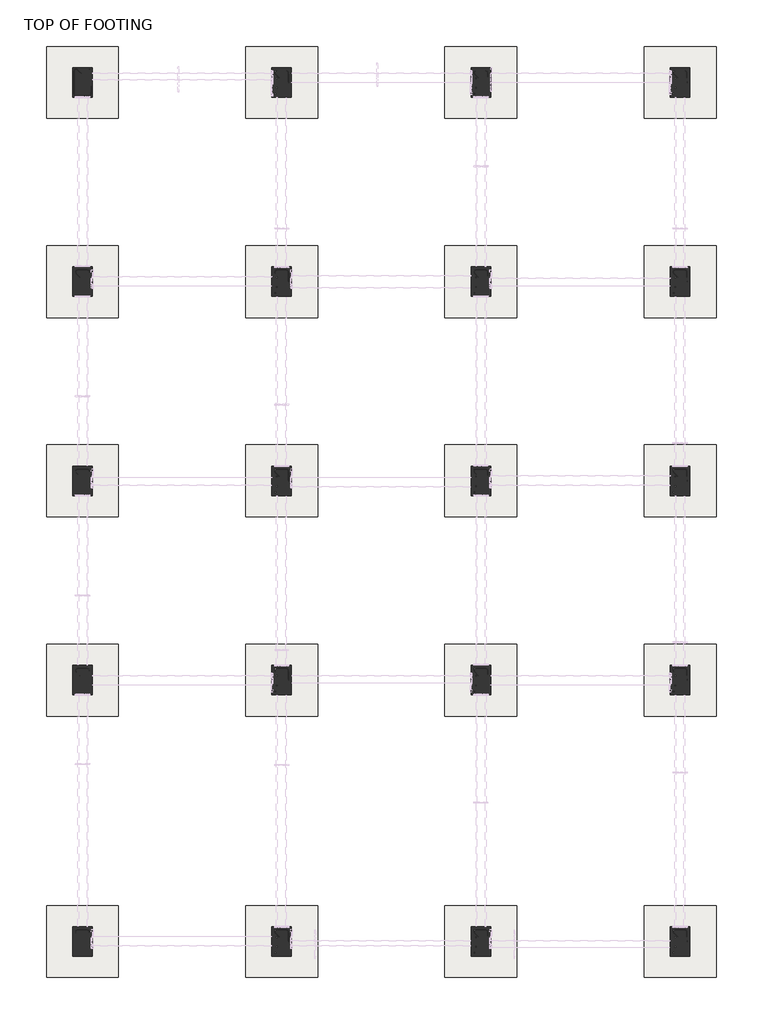
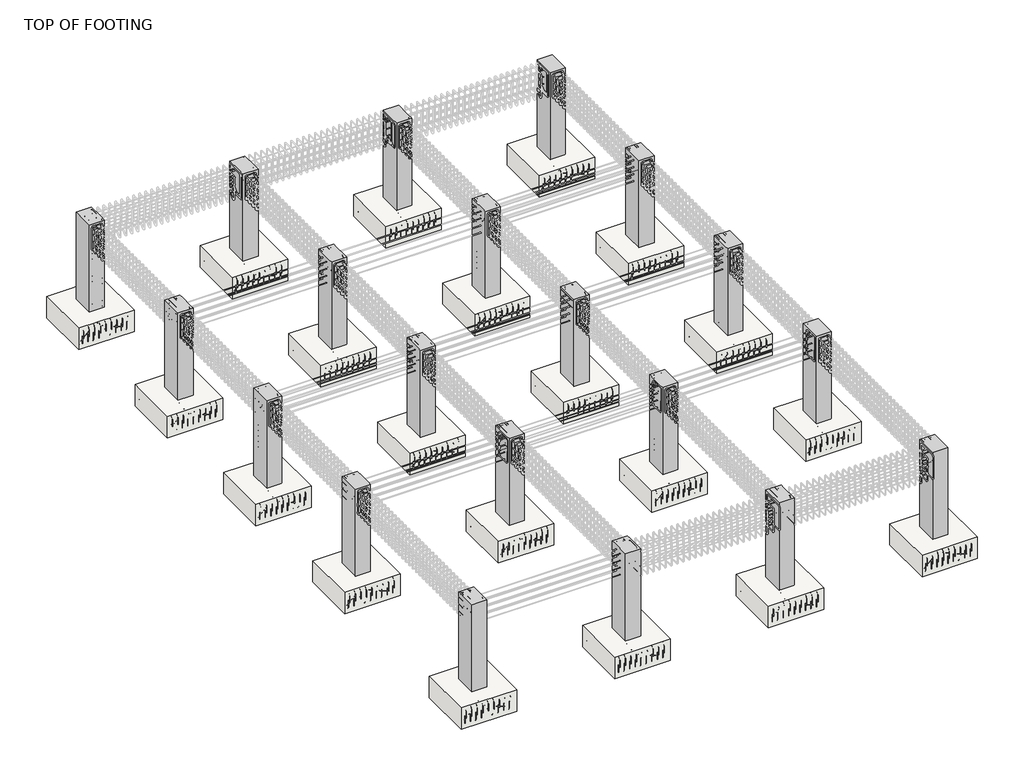
# One storey, part 1 of 18: 20 columns, 20 slabs.
"""IFC4 building model written with IfcOpenShell, lengths in millimetres."""

from ifc_helpers import new_model, si_unit, origin, place, context, project, spatial, faceted_brep, transform, mapped, element, save
from components import m_footing_rectangular_1100mm_x_1100mm_x_450mm_64323a20

model = new_model("IFC4")

# Units and contexts
model_context = context("Model", 3, world=origin())
ifc_project = project(units=[si_unit("LENGTHUNIT", "METRE", prefix="MILLI")], contexts=[model_context])

# Site, building, storey
site = spatial("IfcSite", under=ifc_project)
building = spatial("IfcBuilding", under=site)
storey = spatial("IfcBuildingStorey", under=building, Name="TOP OF FOOTING", Elevation=-1828.8)

# Columns
placement = place(None, origin())
element("IfcColumn", 1, ObjectType="M_Concrete-Rectangular-Column : 300 x 450mm", at=placement, inside=storey, context=model_context, shape_type="Brep", body=[
    faceted_brep([(-10892.3067643, 19025.6598681, -1828.8), (-10892.3067643, 18575.6598681, -1828.8), (-11192.3067643, 18575.6598681, -1828.8), (-11192.3067643, 19025.6598681, -1828.8), (-10892.3067643, 19025.6598681, 0.0), (-10892.3067643, 18725.6598681, 0.0), (-10892.3067643, 18575.6598681, 0.0), (-11192.3067643, 18575.6598681, 0.0), (-11192.3067643, 19025.6598681, 0.0)], [[[0, 1, 2, 3]], [[4, 5, 6, 1, 0]], [[6, 7, 2, 1]], [[7, 8, 3, 2]], [[8, 4, 0, 3]], [[4, 8, 7, 6, 5]]]),
])
element("IfcColumn", 2, ObjectType="M_Concrete-Rectangular-Column : 300 x 450mm", at=placement, inside=storey, context=model_context, shape_type="Brep", body=[
    faceted_brep([(-7844.3067643, 19025.6598681, -1828.8), (-7844.3067643, 18575.6598681, -1828.8), (-8144.3067643, 18575.6598681, -1828.8), (-8144.3067643, 19025.6598681, -1828.8), (-7844.3067643, 19025.6598681, 0.0), (-7844.3067643, 18725.6598681, 0.0), (-7844.3067643, 18575.6598681, 0.0), (-8144.3067643, 18575.6598681, 0.0), (-8144.3067643, 18725.6598681, 0.0), (-8144.3067643, 19025.6598681, 0.0)], [[[0, 1, 2, 3]], [[4, 5, 6, 1, 0]], [[6, 7, 2, 1]], [[7, 8, 9, 3, 2]], [[9, 4, 0, 3]], [[4, 9, 8, 7, 6, 5]]]),
])
element("IfcColumn", 3, ObjectType="M_Concrete-Rectangular-Column : 300 x 450mm", at=placement, inside=storey, context=model_context, shape_type="Brep", body=[
    faceted_brep([(-4796.3067643, 19025.6598681, -1828.8), (-4796.3067643, 18575.6598681, -1828.8), (-5096.3067643, 18575.6598681, -1828.8), (-5096.3067643, 19025.6598681, -1828.8), (-4796.3067643, 19025.6598681, 0.0), (-4796.3067643, 18725.6598681, 0.0), (-4796.3067643, 18575.6598681, 0.0), (-5096.3067643, 18575.6598681, 0.0), (-5096.3067643, 18725.6598681, 0.0), (-5096.3067643, 19025.6598681, 0.0)], [[[0, 1, 2, 3]], [[4, 5, 6, 1, 0]], [[6, 7, 2, 1]], [[7, 8, 9, 3, 2]], [[9, 4, 0, 3]], [[4, 9, 8, 7, 6, 5]]]),
])
element("IfcColumn", 4, ObjectType="M_Concrete-Rectangular-Column : 300 x 450mm", at=placement, inside=storey, context=model_context, shape_type="Brep", body=[
    faceted_brep([(-1748.3067643, 19025.6598681, -1828.8), (-1748.3067643, 18575.6598681, -1828.8), (-2048.3067643, 18575.6598681, -1828.8), (-2048.3067643, 19025.6598681, -1828.8), (-1748.3067643, 19025.6598681, 0.0), (-1748.3067643, 18575.6598681, 0.0), (-2048.3067643, 18575.6598681, 0.0), (-2048.3067643, 18725.6598681, 0.0), (-2048.3067643, 19025.6598681, 0.0)], [[[0, 1, 2, 3]], [[4, 5, 1, 0]], [[5, 6, 2, 1]], [[6, 7, 8, 3, 2]], [[8, 4, 0, 3]], [[4, 8, 7, 6, 5]]]),
])
element("IfcColumn", 5, ObjectType="M_Concrete-Rectangular-Column : 300 x 450mm", at=placement, inside=storey, context=model_context, shape_type="Brep", body=[
    faceted_brep([(-1748.3067643, 15977.6598681, -1828.8), (-1748.3067643, 15527.6598681, -1828.8), (-2048.3067643, 15527.6598681, -1828.8), (-2048.3067643, 15977.6598681, -1828.8), (-1748.3067643, 15977.6598681, 0.0), (-1748.3067643, 15527.6598681, 0.0), (-2048.3067643, 15527.6598681, 0.0), (-2048.3067643, 15602.6598681, 0.0), (-2048.3067643, 15902.6598681, 0.0), (-2048.3067643, 15977.6598681, 0.0)], [[[0, 1, 2, 3]], [[4, 5, 1, 0]], [[5, 6, 2, 1]], [[6, 7, 8, 9, 3, 2]], [[9, 4, 0, 3]], [[4, 9, 8, 7, 6, 5]]]),
])
element("IfcColumn", 6, ObjectType="M_Concrete-Rectangular-Column : 300 x 450mm", at=placement, inside=storey, context=model_context, shape_type="Brep", body=[
    faceted_brep([(-4796.3067643, 15977.6598681, -1828.8), (-4796.3067643, 15527.6598681, -1828.8), (-5096.3067643, 15527.6598681, -1828.8), (-5096.3067643, 15977.6598681, -1828.8), (-4796.3067643, 15977.6598681, 0.0), (-4796.3067643, 15902.6598681, 0.0), (-4796.3067643, 15602.6598681, 0.0), (-4796.3067643, 15527.6598681, 0.0), (-5096.3067643, 15527.6598681, 0.0), (-5096.3067643, 15602.6598681, 0.0), (-5096.3067643, 15902.6598681, 0.0), (-5096.3067643, 15977.6598681, 0.0)], [[[0, 1, 2, 3]], [[4, 5, 6, 7, 1, 0]], [[7, 8, 2, 1]], [[8, 9, 10, 11, 3, 2]], [[11, 4, 0, 3]], [[4, 11, 10, 9, 8, 7, 6, 5]]]),
])
element("IfcColumn", 7, ObjectType="M_Concrete-Rectangular-Column : 300 x 450mm", at=placement, inside=storey, context=model_context, shape_type="Brep", body=[
    faceted_brep([(-7844.3067643, 15977.6598681, -1828.8), (-7844.3067643, 15527.6598681, -1828.8), (-8144.3067643, 15527.6598681, -1828.8), (-8144.3067643, 15977.6598681, -1828.8), (-7844.3067643, 15977.6598681, 0.0), (-7844.3067643, 15902.6598681, 0.0), (-7844.3067643, 15602.6598681, 0.0), (-7844.3067643, 15527.6598681, 0.0), (-8144.3067643, 15527.6598681, 0.0), (-8144.3067643, 15602.6598681, 0.0), (-8144.3067643, 15902.6598681, 0.0), (-8144.3067643, 15977.6598681, 0.0)], [[[0, 1, 2, 3]], [[4, 5, 6, 7, 1, 0]], [[7, 8, 2, 1]], [[8, 9, 10, 11, 3, 2]], [[11, 4, 0, 3]], [[4, 11, 10, 9, 8, 7, 6, 5]]]),
])
element("IfcColumn", 8, ObjectType="M_Concrete-Rectangular-Column : 300 x 450mm", at=placement, inside=storey, context=model_context, shape_type="Brep", body=[
    faceted_brep([(-10892.3067643, 15977.6598681, -1828.8), (-10892.3067643, 15527.6598681, -1828.8), (-11192.3067643, 15527.6598681, -1828.8), (-11192.3067643, 15977.6598681, -1828.8), (-10892.3067643, 15977.6598681, 0.0), (-10892.3067643, 15902.6598681, 0.0), (-10892.3067643, 15602.6598681, 0.0), (-10892.3067643, 15527.6598681, 0.0), (-11192.3067643, 15527.6598681, 0.0), (-11192.3067643, 15977.6598681, 0.0)], [[[0, 1, 2, 3]], [[4, 5, 6, 7, 1, 0]], [[7, 8, 2, 1]], [[8, 9, 3, 2]], [[9, 4, 0, 3]], [[4, 9, 8, 7, 6, 5]]]),
])
element("IfcColumn", 9, ObjectType="M_Concrete-Rectangular-Column : 300 x 450mm", at=placement, inside=storey, context=model_context, shape_type="Brep", body=[
    faceted_brep([(-10892.3067643, 12929.6598681, -1828.8), (-10892.3067643, 12479.6598681, -1828.8), (-11192.3067643, 12479.6598681, -1828.8), (-11192.3067643, 12929.6598681, -1828.8), (-10892.3067643, 12929.6598681, 0.0), (-10892.3067643, 12779.6598681, 0.0), (-10892.3067643, 12554.6598681, 0.0), (-10892.3067643, 12479.6598681, 0.0), (-11192.3067643, 12479.6598681, 0.0), (-11192.3067643, 12929.6598681, 0.0)], [[[0, 1, 2, 3]], [[4, 5, 6, 7, 1, 0]], [[7, 8, 2, 1]], [[8, 9, 3, 2]], [[9, 4, 0, 3]], [[4, 9, 8, 7, 6, 5]]]),
])
element("IfcColumn", 10, ObjectType="M_Concrete-Rectangular-Column : 300 x 450mm", at=placement, inside=storey, context=model_context, shape_type="Brep", body=[
    faceted_brep([(-7844.3067643, 12929.6598681, -1828.8), (-7844.3067643, 12479.6598681, -1828.8), (-8144.3067643, 12479.6598681, -1828.8), (-8144.3067643, 12929.6598681, -1828.8), (-7844.3067643, 12929.6598681, 0.0), (-7844.3067643, 12779.6598681, 0.0), (-7844.3067643, 12554.6598681, 0.0), (-7844.3067643, 12479.6598681, 0.0), (-8144.3067643, 12479.6598681, 0.0), (-8144.3067643, 12554.6598681, 0.0), (-8144.3067643, 12779.6598681, 0.0), (-8144.3067643, 12929.6598681, 0.0)], [[[0, 1, 2, 3]], [[4, 5, 6, 7, 1, 0]], [[7, 8, 2, 1]], [[8, 9, 10, 11, 3, 2]], [[11, 4, 0, 3]], [[4, 11, 10, 9, 8, 7, 6, 5]]]),
])
element("IfcColumn", 11, ObjectType="M_Concrete-Rectangular-Column : 300 x 450mm", at=placement, inside=storey, context=model_context, shape_type="Brep", body=[
    faceted_brep([(-4796.3067643, 12929.6598681, -1828.8), (-4796.3067643, 12479.6598681, -1828.8), (-5096.3067643, 12479.6598681, -1828.8), (-5096.3067643, 12929.6598681, -1828.8), (-4796.3067643, 12929.6598681, 0.0), (-4796.3067643, 12779.6598681, 0.0), (-4796.3067643, 12554.6598681, 0.0), (-4796.3067643, 12479.6598681, 0.0), (-5096.3067643, 12479.6598681, 0.0), (-5096.3067643, 12554.6598681, 0.0), (-5096.3067643, 12779.6598681, 0.0), (-5096.3067643, 12929.6598681, 0.0)], [[[0, 1, 2, 3]], [[4, 5, 6, 7, 1, 0]], [[7, 8, 2, 1]], [[8, 9, 10, 11, 3, 2]], [[11, 4, 0, 3]], [[4, 11, 10, 9, 8, 7, 6, 5]]]),
])
element("IfcColumn", 12, ObjectType="M_Concrete-Rectangular-Column : 300 x 450mm", at=placement, inside=storey, context=model_context, shape_type="Brep", body=[
    faceted_brep([(-1748.3067643, 12929.6598681, -1828.8), (-1748.3067643, 12479.6598681, -1828.8), (-2048.3067643, 12479.6598681, -1828.8), (-2048.3067643, 12929.6598681, -1828.8), (-1748.3067643, 12929.6598681, 0.0), (-1748.3067643, 12479.6598681, 0.0), (-2048.3067643, 12479.6598681, 0.0), (-2048.3067643, 12554.6598681, 0.0), (-2048.3067643, 12779.6598681, 0.0), (-2048.3067643, 12929.6598681, 0.0)], [[[0, 1, 2, 3]], [[4, 5, 1, 0]], [[5, 6, 2, 1]], [[6, 7, 8, 9, 3, 2]], [[9, 4, 0, 3]], [[4, 9, 8, 7, 6, 5]]]),
])
element("IfcColumn", 13, ObjectType="M_Concrete-Rectangular-Column : 300 x 450mm", at=placement, inside=storey, context=model_context, shape_type="Brep", body=[
    faceted_brep([(-1748.3067643, 9881.6598681, -1828.8), (-1748.3067643, 9431.6598681, -1828.8), (-2048.3067643, 9431.6598681, -1828.8), (-2048.3067643, 9881.6598681, -1828.8), (-1748.3067643, 9881.6598681, 0.0), (-1748.3067643, 9431.6598681, 0.0), (-2048.3067643, 9431.6598681, 0.0), (-2048.3067643, 9506.6598681, 0.0), (-2048.3067643, 9731.6598681, 0.0), (-2048.3067643, 9881.6598681, 0.0)], [[[0, 1, 2, 3]], [[4, 5, 1, 0]], [[5, 6, 2, 1]], [[6, 7, 8, 9, 3, 2]], [[9, 4, 0, 3]], [[4, 9, 8, 7, 6, 5]]]),
])
element("IfcColumn", 14, ObjectType="M_Concrete-Rectangular-Column : 300 x 450mm", at=placement, inside=storey, context=model_context, shape_type="Brep", body=[
    faceted_brep([(-4796.3067643, 9881.6598681, -1828.8), (-4796.3067643, 9431.6598681, -1828.8), (-5096.3067643, 9431.6598681, -1828.8), (-5096.3067643, 9881.6598681, -1828.8), (-4796.3067643, 9881.6598681, 0.0), (-4796.3067643, 9731.6598681, 0.0), (-4796.3067643, 9506.6598681, 0.0), (-4796.3067643, 9431.6598681, 0.0), (-5096.3067643, 9431.6598681, 0.0), (-5096.3067643, 9506.6598681, 0.0), (-5096.3067643, 9731.6598681, 0.0), (-5096.3067643, 9881.6598681, 0.0)], [[[0, 1, 2, 3]], [[4, 5, 6, 7, 1, 0]], [[7, 8, 2, 1]], [[8, 9, 10, 11, 3, 2]], [[11, 4, 0, 3]], [[4, 11, 10, 9, 8, 7, 6, 5]]]),
])
element("IfcColumn", 15, ObjectType="M_Concrete-Rectangular-Column : 300 x 450mm", at=placement, inside=storey, context=model_context, shape_type="Brep", body=[
    faceted_brep([(-7844.3067643, 9881.6598681, -1828.8), (-7844.3067643, 9431.6598681, -1828.8), (-8144.3067643, 9431.6598681, -1828.8), (-8144.3067643, 9881.6598681, -1828.8), (-7844.3067643, 9881.6598681, 0.0), (-7844.3067643, 9731.6598681, 0.0), (-7844.3067643, 9506.6598681, 0.0), (-7844.3067643, 9431.6598681, 0.0), (-8144.3067643, 9431.6598681, 0.0), (-8144.3067643, 9506.6598681, 0.0), (-8144.3067643, 9731.6598681, 0.0), (-8144.3067643, 9881.6598681, 0.0)], [[[0, 1, 2, 3]], [[4, 5, 6, 7, 1, 0]], [[7, 8, 2, 1]], [[8, 9, 10, 11, 3, 2]], [[11, 4, 0, 3]], [[4, 11, 10, 9, 8, 7, 6, 5]]]),
])
element("IfcColumn", 16, ObjectType="M_Concrete-Rectangular-Column : 300 x 450mm", at=placement, inside=storey, context=model_context, shape_type="Brep", body=[
    faceted_brep([(-10892.3067643, 9881.6598681, -1828.8), (-10892.3067643, 9431.6598681, -1828.8), (-11192.3067643, 9431.6598681, -1828.8), (-11192.3067643, 9881.6598681, -1828.8), (-10892.3067643, 9881.6598681, 0.0), (-10892.3067643, 9731.6598681, 0.0), (-10892.3067643, 9506.6598681, 0.0), (-10892.3067643, 9431.6598681, 0.0), (-11192.3067643, 9431.6598681, 0.0), (-11192.3067643, 9881.6598681, 0.0)], [[[0, 1, 2, 3]], [[4, 5, 6, 7, 1, 0]], [[7, 8, 2, 1]], [[8, 9, 3, 2]], [[9, 4, 0, 3]], [[4, 9, 8, 7, 6, 5]]]),
])
element("IfcColumn", 17, ObjectType="M_Concrete-Rectangular-Column : 300 x 450mm", at=placement, inside=storey, context=model_context, shape_type="Brep", body=[
    faceted_brep([(-10892.3067643, 5881.6598681, -1828.8), (-10892.3067643, 5431.6598681, -1828.8), (-11192.3067643, 5431.6598681, -1828.8), (-11192.3067643, 5881.6598681, -1828.8), (-10892.3067643, 5881.6598681, 0.0), (-10892.3067643, 5806.6598681, 0.0), (-10892.3067643, 5431.6598681, 0.0), (-11192.3067643, 5431.6598681, 0.0), (-11192.3067643, 5881.6598681, 0.0)], [[[0, 1, 2, 3]], [[4, 5, 6, 1, 0]], [[6, 7, 2, 1]], [[7, 8, 3, 2]], [[8, 4, 0, 3]], [[4, 8, 7, 6, 5]]]),
])
element("IfcColumn", 18, ObjectType="M_Concrete-Rectangular-Column : 300 x 450mm", at=placement, inside=storey, context=model_context, shape_type="Brep", body=[
    faceted_brep([(-7844.3067643, 5881.6598681, -1828.8), (-7844.3067643, 5431.6598681, -1828.8), (-8144.3067643, 5431.6598681, -1828.8), (-8144.3067643, 5881.6598681, -1828.8), (-7844.3067643, 5881.6598681, 0.0), (-7844.3067643, 5806.6598681, 0.0), (-7844.3067643, 5431.6598681, 0.0), (-8144.3067643, 5431.6598681, 0.0), (-8144.3067643, 5806.6598681, 0.0), (-8144.3067643, 5881.6598681, 0.0)], [[[0, 1, 2, 3]], [[4, 5, 6, 1, 0]], [[6, 7, 2, 1]], [[7, 8, 9, 3, 2]], [[9, 4, 0, 3]], [[4, 9, 8, 7, 6, 5]]]),
])
element("IfcColumn", 19, ObjectType="M_Concrete-Rectangular-Column : 300 x 450mm", at=placement, inside=storey, context=model_context, shape_type="Brep", body=[
    faceted_brep([(-4796.3067643, 5881.6598681, -1828.8), (-4796.3067643, 5431.6598681, -1828.8), (-5096.3067643, 5431.6598681, -1828.8), (-5096.3067643, 5881.6598681, -1828.8), (-4796.3067643, 5881.6598681, 0.0), (-4796.3067643, 5806.6598681, 0.0), (-4796.3067643, 5431.6598681, 0.0), (-5096.3067643, 5431.6598681, 0.0), (-5096.3067643, 5806.6598681, 0.0), (-5096.3067643, 5881.6598681, 0.0)], [[[0, 1, 2, 3]], [[4, 5, 6, 1, 0]], [[6, 7, 2, 1]], [[7, 8, 9, 3, 2]], [[9, 4, 0, 3]], [[4, 9, 8, 7, 6, 5]]]),
])
element("IfcColumn", 20, ObjectType="M_Concrete-Rectangular-Column : 300 x 450mm", at=placement, inside=storey, context=model_context, shape_type="Brep", body=[
    faceted_brep([(-1748.3067643, 5881.6598681, -1828.8), (-1748.3067643, 5431.6598681, -1828.8), (-2048.3067643, 5431.6598681, -1828.8), (-2048.3067643, 5881.6598681, -1828.8), (-1748.3067643, 5881.6598681, 0.0), (-1748.3067643, 5431.6598681, 0.0), (-2048.3067643, 5431.6598681, 0.0), (-2048.3067643, 5806.6598681, 0.0), (-2048.3067643, 5881.6598681, 0.0)], [[[0, 1, 2, 3]], [[4, 5, 1, 0]], [[5, 6, 2, 1]], [[6, 7, 8, 3, 2]], [[8, 4, 0, 3]], [[4, 8, 7, 6, 5]]]),
])

# Slabs
m_footing_rectangular_1100mm_x_1100mm_x_450mm_shape = m_footing_rectangular_1100mm_x_1100mm_x_450mm_64323a20(model_context)
element("IfcSlab", 21, ObjectType="M_Footing-Rectangular : 1100MM X 1100MM X 450MM", at=placement, inside=storey, context=model_context, shape_type="MappedRepresentation", body=[
    mapped(m_footing_rectangular_1100mm_x_1100mm_x_450mm_shape, transform((-11042.3067643, 18800.6598681, -1828.8), x_axis=(1.0, 0.0, 0.0), y_axis=(0.0, 1.0, 0.0), z_axis=(0.0, 0.0, 1.0))),
])
element("IfcSlab", 22, ObjectType="M_Footing-Rectangular : 1100MM X 1100MM X 450MM", at=placement, inside=storey, context=model_context, shape_type="MappedRepresentation", body=[
    mapped(m_footing_rectangular_1100mm_x_1100mm_x_450mm_shape, transform((-7994.3067643, 18800.6598681, -1828.8), x_axis=(1.0, 0.0, 0.0), y_axis=(0.0, 1.0, 0.0), z_axis=(0.0, 0.0, 1.0))),
])
element("IfcSlab", 23, ObjectType="M_Footing-Rectangular : 1100MM X 1100MM X 450MM", at=placement, inside=storey, context=model_context, shape_type="MappedRepresentation", body=[
    mapped(m_footing_rectangular_1100mm_x_1100mm_x_450mm_shape, transform((-4946.3067643, 18800.6598681, -1828.8), x_axis=(1.0, 0.0, 0.0), y_axis=(0.0, 1.0, 0.0), z_axis=(0.0, 0.0, 1.0))),
])
element("IfcSlab", 24, ObjectType="M_Footing-Rectangular : 1100MM X 1100MM X 450MM", at=placement, inside=storey, context=model_context, shape_type="MappedRepresentation", body=[
    mapped(m_footing_rectangular_1100mm_x_1100mm_x_450mm_shape, transform((-1898.3067643, 18800.6598681, -1828.8), x_axis=(1.0, 0.0, 0.0), y_axis=(0.0, 1.0, 0.0), z_axis=(0.0, 0.0, 1.0))),
])
element("IfcSlab", 25, ObjectType="M_Footing-Rectangular : 1100MM X 1100MM X 450MM", at=placement, inside=storey, context=model_context, shape_type="MappedRepresentation", body=[
    mapped(m_footing_rectangular_1100mm_x_1100mm_x_450mm_shape, transform((-1898.3067643, 15752.6598681, -1828.8), x_axis=(1.0, 0.0, 0.0), y_axis=(0.0, 1.0, 0.0), z_axis=(0.0, 0.0, 1.0))),
])
element("IfcSlab", 26, ObjectType="M_Footing-Rectangular : 1100MM X 1100MM X 450MM", at=placement, inside=storey, context=model_context, shape_type="MappedRepresentation", body=[
    mapped(m_footing_rectangular_1100mm_x_1100mm_x_450mm_shape, transform((-4946.3067643, 15752.6598681, -1828.8), x_axis=(1.0, 0.0, 0.0), y_axis=(0.0, 1.0, 0.0), z_axis=(0.0, 0.0, 1.0))),
])
element("IfcSlab", 27, ObjectType="M_Footing-Rectangular : 1100MM X 1100MM X 450MM", at=placement, inside=storey, context=model_context, shape_type="MappedRepresentation", body=[
    mapped(m_footing_rectangular_1100mm_x_1100mm_x_450mm_shape, transform((-7994.3067643, 15752.6598681, -1828.8), x_axis=(1.0, 0.0, 0.0), y_axis=(0.0, 1.0, 0.0), z_axis=(0.0, 0.0, 1.0))),
])
element("IfcSlab", 28, ObjectType="M_Footing-Rectangular : 1100MM X 1100MM X 450MM", at=placement, inside=storey, context=model_context, shape_type="MappedRepresentation", body=[
    mapped(m_footing_rectangular_1100mm_x_1100mm_x_450mm_shape, transform((-11042.3067643, 15752.6598681, -1828.8), x_axis=(1.0, 0.0, 0.0), y_axis=(0.0, 1.0, 0.0), z_axis=(0.0, 0.0, 1.0))),
])
element("IfcSlab", 29, ObjectType="M_Footing-Rectangular : 1100MM X 1100MM X 450MM", at=placement, inside=storey, context=model_context, shape_type="MappedRepresentation", body=[
    mapped(m_footing_rectangular_1100mm_x_1100mm_x_450mm_shape, transform((-11042.3067643, 12704.6598681, -1828.8), x_axis=(1.0, 0.0, 0.0), y_axis=(0.0, 1.0, 0.0), z_axis=(0.0, 0.0, 1.0))),
])
element("IfcSlab", 30, ObjectType="M_Footing-Rectangular : 1100MM X 1100MM X 450MM", at=placement, inside=storey, context=model_context, shape_type="MappedRepresentation", body=[
    mapped(m_footing_rectangular_1100mm_x_1100mm_x_450mm_shape, transform((-7994.3067643, 12704.6598681, -1828.8), x_axis=(1.0, 0.0, 0.0), y_axis=(0.0, 1.0, 0.0), z_axis=(0.0, 0.0, 1.0))),
])
element("IfcSlab", 31, ObjectType="M_Footing-Rectangular : 1100MM X 1100MM X 450MM", at=placement, inside=storey, context=model_context, shape_type="MappedRepresentation", body=[
    mapped(m_footing_rectangular_1100mm_x_1100mm_x_450mm_shape, transform((-4946.3067643, 12704.6598681, -1828.8), x_axis=(1.0, 0.0, 0.0), y_axis=(0.0, 1.0, 0.0), z_axis=(0.0, 0.0, 1.0))),
])
element("IfcSlab", 32, ObjectType="M_Footing-Rectangular : 1100MM X 1100MM X 450MM", at=placement, inside=storey, context=model_context, shape_type="MappedRepresentation", body=[
    mapped(m_footing_rectangular_1100mm_x_1100mm_x_450mm_shape, transform((-1898.3067643, 12704.6598681, -1828.8), x_axis=(1.0, 0.0, 0.0), y_axis=(0.0, 1.0, 0.0), z_axis=(0.0, 0.0, 1.0))),
])
element("IfcSlab", 33, ObjectType="M_Footing-Rectangular : 1100MM X 1100MM X 450MM", at=placement, inside=storey, context=model_context, shape_type="MappedRepresentation", body=[
    mapped(m_footing_rectangular_1100mm_x_1100mm_x_450mm_shape, transform((-1898.3067643, 9656.6598681, -1828.8), x_axis=(1.0, 0.0, 0.0), y_axis=(0.0, 1.0, 0.0), z_axis=(0.0, 0.0, 1.0))),
])
element("IfcSlab", 34, ObjectType="M_Footing-Rectangular : 1100MM X 1100MM X 450MM", at=placement, inside=storey, context=model_context, shape_type="MappedRepresentation", body=[
    mapped(m_footing_rectangular_1100mm_x_1100mm_x_450mm_shape, transform((-4946.3067643, 9656.6598681, -1828.8), x_axis=(1.0, 0.0, 0.0), y_axis=(0.0, 1.0, 0.0), z_axis=(0.0, 0.0, 1.0))),
])
element("IfcSlab", 35, ObjectType="M_Footing-Rectangular : 1100MM X 1100MM X 450MM", at=placement, inside=storey, context=model_context, shape_type="MappedRepresentation", body=[
    mapped(m_footing_rectangular_1100mm_x_1100mm_x_450mm_shape, transform((-7994.3067643, 9656.6598681, -1828.8), x_axis=(1.0, 0.0, 0.0), y_axis=(0.0, 1.0, 0.0), z_axis=(0.0, 0.0, 1.0))),
])
element("IfcSlab", 36, ObjectType="M_Footing-Rectangular : 1100MM X 1100MM X 450MM", at=placement, inside=storey, context=model_context, shape_type="MappedRepresentation", body=[
    mapped(m_footing_rectangular_1100mm_x_1100mm_x_450mm_shape, transform((-11042.3067643, 9656.6598681, -1828.8), x_axis=(1.0, 0.0, 0.0), y_axis=(0.0, 1.0, 0.0), z_axis=(0.0, 0.0, 1.0))),
])
element("IfcSlab", 37, ObjectType="M_Footing-Rectangular : 1100MM X 1100MM X 450MM", at=placement, inside=storey, context=model_context, shape_type="MappedRepresentation", body=[
    mapped(m_footing_rectangular_1100mm_x_1100mm_x_450mm_shape, transform((-1898.3067643, 5656.6598681, -1828.8), x_axis=(1.0, 0.0, 0.0), y_axis=(0.0, 1.0, 0.0), z_axis=(0.0, 0.0, 1.0))),
])
element("IfcSlab", 38, ObjectType="M_Footing-Rectangular : 1100MM X 1100MM X 450MM", at=placement, inside=storey, context=model_context, shape_type="MappedRepresentation", body=[
    mapped(m_footing_rectangular_1100mm_x_1100mm_x_450mm_shape, transform((-4946.3067643, 5656.6598681, -1828.8), x_axis=(1.0, 0.0, 0.0), y_axis=(0.0, 1.0, 0.0), z_axis=(0.0, 0.0, 1.0))),
])
element("IfcSlab", 39, ObjectType="M_Footing-Rectangular : 1100MM X 1100MM X 450MM", at=placement, inside=storey, context=model_context, shape_type="MappedRepresentation", body=[
    mapped(m_footing_rectangular_1100mm_x_1100mm_x_450mm_shape, transform((-7994.3067643, 5656.6598681, -1828.8), x_axis=(1.0, 0.0, 0.0), y_axis=(0.0, 1.0, 0.0), z_axis=(0.0, 0.0, 1.0))),
])
element("IfcSlab", 40, ObjectType="M_Footing-Rectangular : 1100MM X 1100MM X 450MM", at=placement, inside=storey, context=model_context, shape_type="MappedRepresentation", body=[
    mapped(m_footing_rectangular_1100mm_x_1100mm_x_450mm_shape, transform((-11042.3067643, 5656.6598681, -1828.8), x_axis=(1.0, 0.0, 0.0), y_axis=(0.0, 1.0, 0.0), z_axis=(0.0, 0.0, 1.0))),
])

save(model, "model.ifc")

# Revit data of these elements
# Grids (mm)
#   "A": line (-11042.307, 22651.047) -> (-11042.307, 3615.495)
#   "B": line (-7994.307, 22651.047) -> (-7994.307, 3615.495)
#   "C": line (-4946.307, 22651.047) -> (-4946.307, 3615.495)
#   "D": line (-1898.307, 22651.047) -> (-1898.307, 3615.495)
#   "1": line (2361.601, 18800.66) -> (-15996.694, 18800.66)
#   "2": line (2361.601, 15752.66) -> (-15996.694, 15752.66)
#   "3": line (2361.601, 12704.66) -> (-15996.694, 12704.66)
#   "4": line (2361.601, 9656.66) -> (-15996.694, 9656.66)
#   "5": line (2361.601, 5656.66) -> (-15996.694, 5656.66)
# Type "M_Concrete-Rectangular-Column : 300 x 450mm"
#   b = 300 mm
#   h = 450 mm
#   Structural Material [instance default] = Concrete, Cast-in-Place gray
# Type "M_Footing-Rectangular : 1100MM X 1100MM X 450MM"
#   Width = 1100 mm
#   Length = 1100 mm
#   Foundation Thickness = 450 mm
#   Structural Material [instance default] = Concrete, Cast-in-Place gray
#   Assembly Code = ""
# Elements 1, 2, 3, 4, 5, 6, 7, 8, 9, 10, 11, 12, 13, 14, 15, 16, 17, 18, 19, 20 (IfcColumn, "M_Concrete-Rectangular-Column : 300 x 450mm")
#   Structural Material = Concrete, Cast-in-Place gray
#   Phase Created = New Construction
#   Materials on its faces: "Concrete, Cast-in-Place gray"
# Elements 21, 22, 23, 24, 25, 26, 27, 28, 29, 30, 31, 32, 33, 34, 35, 36, 37, 38, 39, 40 (IfcSlab, "M_Footing-Rectangular : 1100MM X 1100MM X 450MM")
#   Structural Material = Concrete, Cast-in-Place gray
#   Phase Created = New Construction
#   Materials on its faces: "Concrete, Cast-in-Place gray"
# Materials
#   "Concrete, Cast-in-Place gray": class "Concrete", colour RGB 192 192 192, transparency 0, Description = "Cast-in-place concrete", Cost = 0
